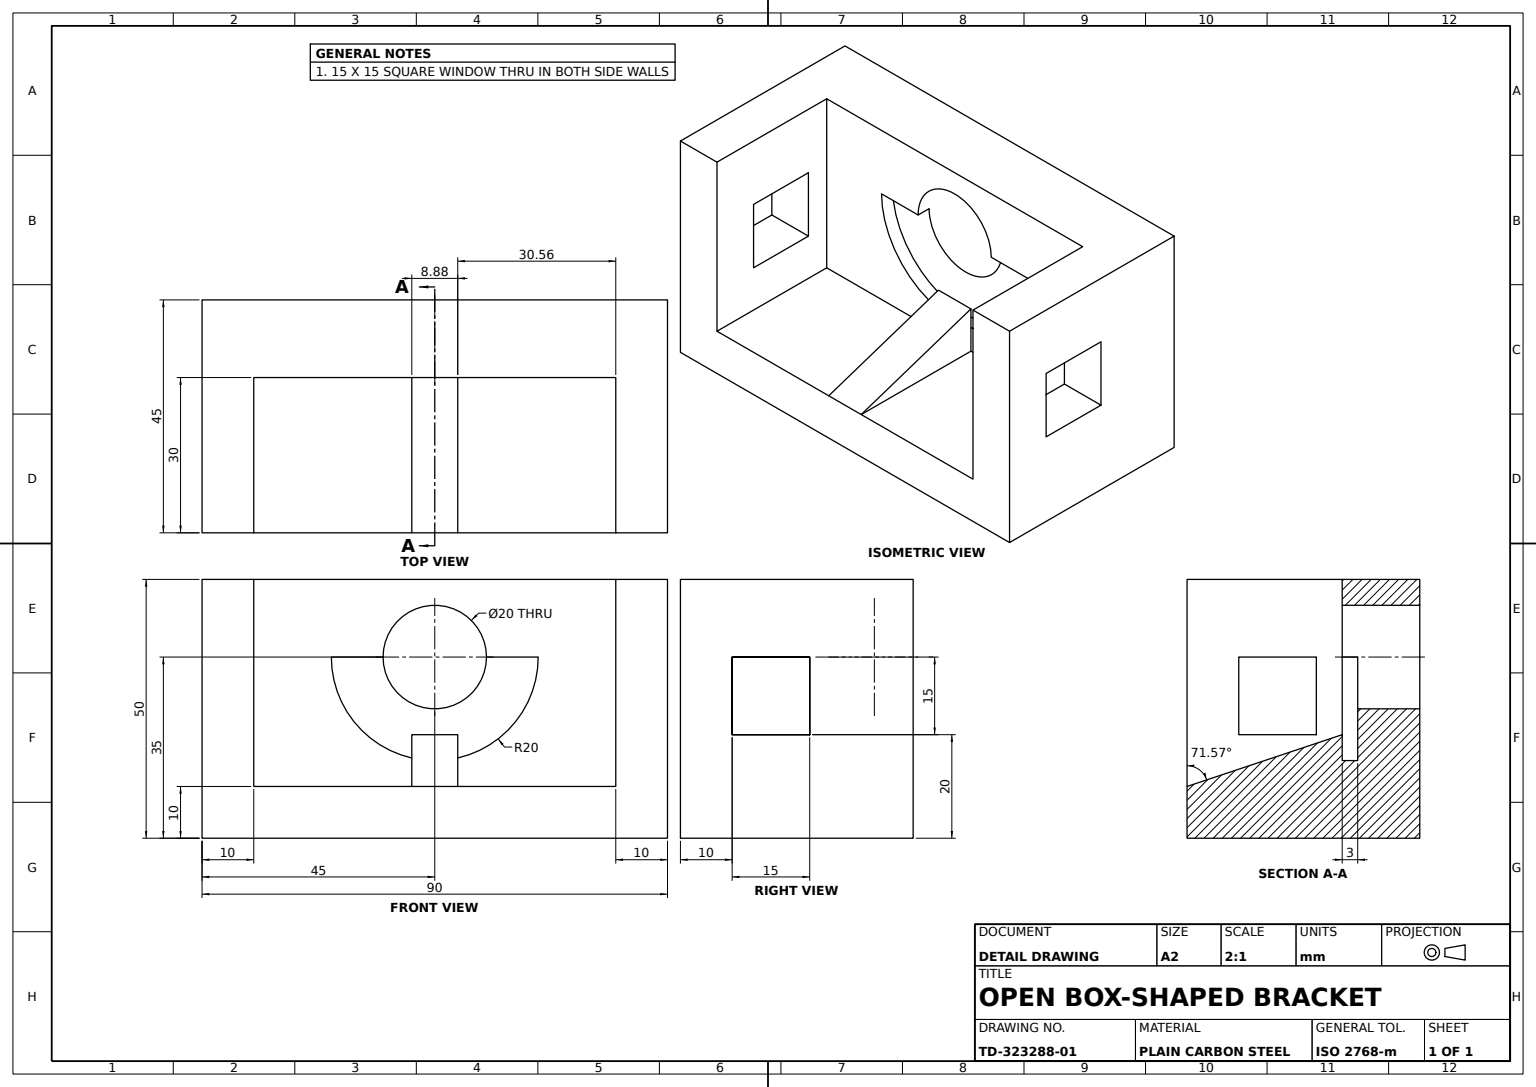
from build123d import *

# Parameters (mm, degrees)
BLOCK_PROFILE_SKETCH_90X50_W   = 90
BLOCK_PROFILE_SKETCH_90X50_H   = 50
BASE_BLOCK_90X50X45_DEPTH      = 45
POCKET_SKETCH_W                = 70
POCKET_SKETCH_H                = 40
INNER_POCKET_30_DEEP_DEPTH     = 30
BORE_SKETCH_R                  = 10
GUIDE_BORE_CUT_DEPTH           = 60.581876439
SIDE_WINDOW_SKETCH_W           = 15
SIDE_WINDOW_SKETCH_H           = 15
SIDE_WINDOWS_15X15_DEPTH       = 104.682206767
RIB_SKETCH_W                   = 8.881329336
RIB_SKETCH_H                   = 10
INTERNAL_RIB_DEPTH             = 30
ARC_RELIEF_GROOVE_3_DEEP_DEPTH = 3
RIB_TRIM_CUT_10_DEEP_DEPTH     = 10


with BuildPart() as part:
    # Block Profile Sketch 90x50 → Base Block 90x50x45 (new body)
    with BuildSketch(Plane.XY):
        Rectangle(BLOCK_PROFILE_SKETCH_90X50_W, BLOCK_PROFILE_SKETCH_90X50_H)
    extrude(amount=-BASE_BLOCK_90X50X45_DEPTH)

    # Pocket Sketch → Inner Pocket 30 Deep (cut)
    with BuildSketch(Plane.XY):
        with Locations((0, 5)):
            Rectangle(POCKET_SKETCH_W, POCKET_SKETCH_H)
    extrude(amount=-INNER_POCKET_30_DEEP_DEPTH, mode=Mode.SUBTRACT)

    # Bore Sketch → Guide Bore Cut (cut, through all)
    with BuildSketch(Plane.XY.offset(-30)):
        with Locations((0, 10)):
            Circle(BORE_SKETCH_R)
    extrude(amount=-GUIDE_BORE_CUT_DEPTH, mode=Mode.SUBTRACT)

    # Side Window Sketch → Side Windows 15x15 (cut, through all)
    with BuildSketch(Plane.ZY.offset(45)):
        with Locations((-17.5, 2.5)):
            Rectangle(SIDE_WINDOW_SKETCH_W, SIDE_WINDOW_SKETCH_H)
    extrude(amount=-SIDE_WINDOWS_15X15_DEPTH, mode=Mode.SUBTRACT)

    # Rib Sketch → Internal Rib (add)
    with BuildSketch(Plane.XY.offset(-30)):
        with Locations((0, -10)):
            Rectangle(RIB_SKETCH_W, RIB_SKETCH_H)
    extrude(amount=INTERNAL_RIB_DEPTH)

    # Arc Groove Sketch → Arc Relief Groove 3 Deep (cut)
    with BuildSketch(Plane.XY.offset(-30)):
        with BuildLine():
            Line((20, 10), (10, 10))
            ThreePointArc((10, 10), (0, 0), (-10, 10))
            Line((-10, 10), (-20, 10))
            ThreePointArc((-20, 10), (0, -10), (20, 10))
        make_face()
    extrude(amount=-ARC_RELIEF_GROOVE_3_DEEP_DEPTH, mode=Mode.SUBTRACT)

    # Rib Trim Sketch → Rib Trim Cut 10 Deep (cut)
    with BuildSketch(Plane(origin=(4.440664668, 0, 0), x_dir=(0, 0, -1), z_dir=(1, 0, 0))):
        Polygon((30, -5), (0, -5), (0, -15), align=None)
    extrude(amount=-RIB_TRIM_CUT_10_DEEP_DEPTH, mode=Mode.SUBTRACT)


solid = part.part
